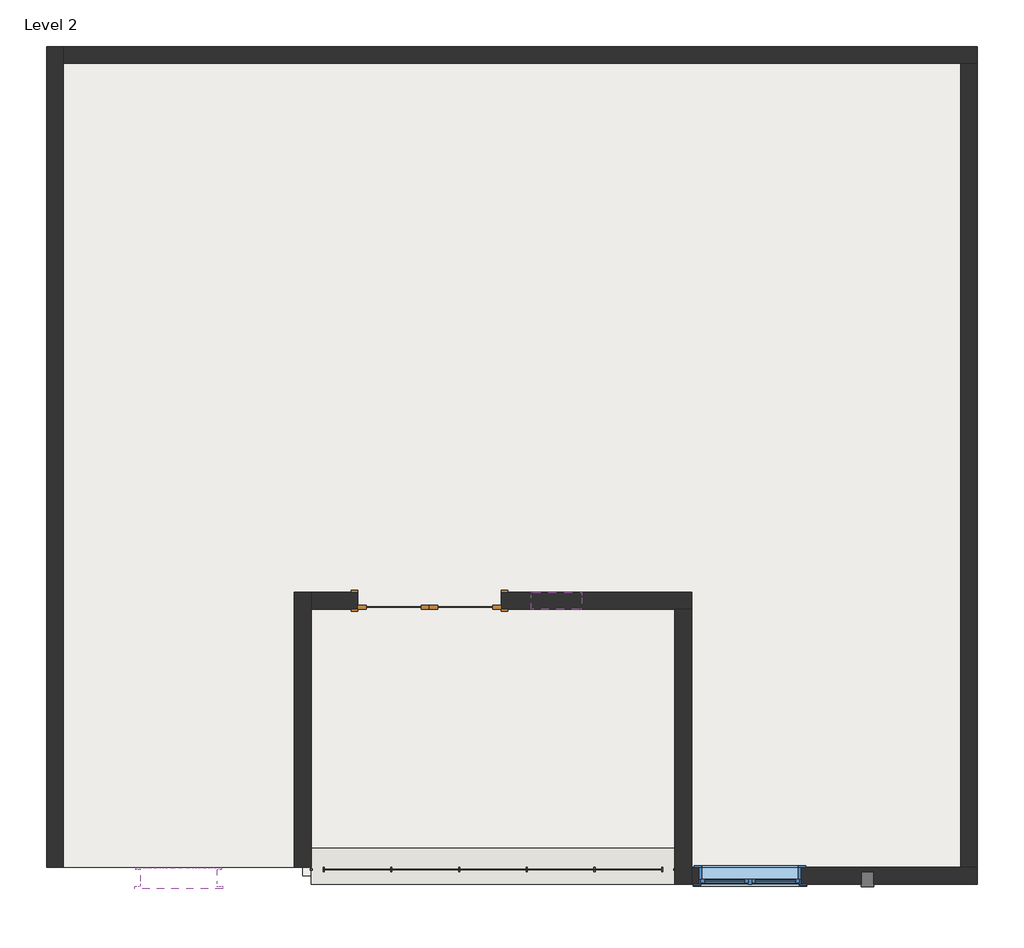
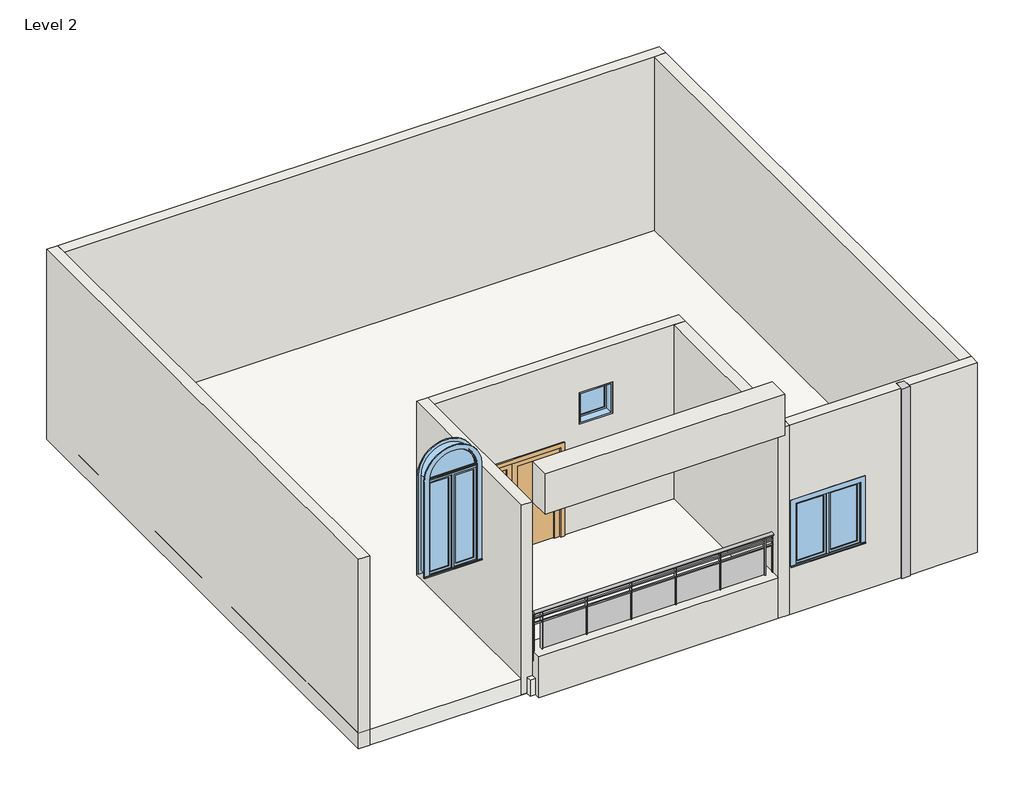
# One storey: 8 walls, 3 windows, 1 door, 1 proxy, 1 railing, 1 roof.
"""IFC4 building model written with IfcOpenShell, lengths in millimetres."""

from ifc_helpers import new_model, si_unit, point, frame, origin, place, context, project, spatial, polyline, ellipse_curve, trimmed, outline, extrude, faceted_brep, transform, mapped, element, save
from ifc_brep_helpers import plane_surface, extruded_surface, advanced_brep
from components import door_10418eaf, walls_4_walls_4_ee6bbb79, window_4e95f2a8, window_0862ab64, window_6846e476

model = new_model("IFC4")

# Units and contexts
model_context = context("Model", 3, world=origin())
ifc_project = project(units=[si_unit("LENGTHUNIT", "METRE", prefix="MILLI")], contexts=[model_context])

# Site, building, storey
site = spatial("IfcSite", under=ifc_project)
building = spatial("IfcBuilding", under=site)
storey = spatial("IfcBuildingStorey", under=building, Name="Level 2", Elevation=3657.6)

# Proxy
placement = place(None, origin())
element("IfcBuildingElementProxy", 1, Name="Reveal", ObjectType="Reveal", at=placement, inside=storey, context=model_context, shape_type="SweptSolid", body=[
    extrude(outline(polyline([(752.5001186, 242.2810824), (752.5001186, 425.1610824), (904.9001186, 425.1610824), (904.9001186, 242.2810824), (752.5001186, 242.2810824)])), frame((0.0, 0.0, 3657.6), z_axis=(0.0, 0.0, 1.0), x_axis=(1.0, 0.0, 0.0)), (0.0, 0.0, 1.0), 3657.6),
])

# Door
door_shape = door_10418eaf(model_context)
element("IfcDoor", 2, ObjectType="Door-Double-Glass : 68\" x 80\"", at=placement, inside=storey, context=model_context, shape_type="MappedRepresentation", body=[
    mapped(door_shape, transform((-4429.0998814, 3678.7423324, 3657.6), x_axis=(-1.0, 0.0, 0.0), y_axis=(0.0, -1.0, 0.0), z_axis=(0.0, 0.0, 1.0))),
])

# Railing
element("IfcRailing", 3, ObjectType="Glass Panel - Bottom Fill", at=placement, inside=storey, context=model_context, shape_type="SolidModel", body=[
    advanced_brep(
    [(-5851.4998814, 488.6610824, 5181.6), (-5851.4998814, 412.4610824, 5181.6), (-1482.6998814, 488.6610824, 5181.6), (-1482.6998814, 412.4610824, 5181.6)],
    [
        (0, 1, ellipse_curve(frame((-5851.4998814, 450.5610824, 5181.6), z_axis=(-1.0, 0.0, 0.0), x_axis=(0.0, -1.0, 0.0)), 38.1, 28.575)),
        (1, 0, ellipse_curve(frame((-5851.4998814, 450.5610824, 5181.6), z_axis=(-1.0, 0.0, 0.0), x_axis=(0.0, -1.0, 0.0)), 38.1, 28.575)),
        (2, 3, ellipse_curve(frame((-1482.6998814, 450.5610824, 5181.6), z_axis=(1.0, 0.0, 0.0), x_axis=(0.0, -1.0, 0.0)), 38.1, 28.575)),
        (3, 2, ellipse_curve(frame((-1482.6998814, 450.5610824, 5181.6), z_axis=(1.0, 0.0, 0.0), x_axis=(0.0, -1.0, 0.0)), 38.1, 28.575)),
        (0, 2),
        (3, 1),
    ],
    [
        plane_surface(frame((-5851.4998814, 450.5610824, 5181.6), z_axis=(-1.0, 0.0, 0.0), x_axis=(0.0, 1.0, 0.0))),
        plane_surface(frame((-1482.6998814, 450.5610824, 5181.6), z_axis=(1.0, 0.0, 0.0), x_axis=(0.0, 1.0, 0.0))),
        extruded_surface(trimmed(ellipse_curve(frame((-1482.6998814, 450.5610824, 5181.6), z_axis=(-1.0, 0.0, 0.0), x_axis=(0.0, -1.0, 0.0)), 38.1, 28.575), [point((-1482.6998814, 488.6610824, 5181.6))], [point((-1482.6998814, 412.4610824, 5181.6))], True, "CARTESIAN"), (-4368.8, 0.0, 0.0), 4368.8),
        extruded_surface(trimmed(ellipse_curve(frame((-1482.6998814, 450.5610824, 5181.6), z_axis=(-1.0, 0.0, 0.0), x_axis=(0.0, -1.0, 0.0)), 38.1, 28.575), [point((-1482.6998814, 412.4610824, 5181.6))], [point((-1482.6998814, 488.6610824, 5181.6))], True, "CARTESIAN"), (-4368.8, 0.0, 0.0), 4368.8),
    ],
    [
        (0, [[1, 2]]),
        (1, [[3, 4]]),
        (2, [[-1, 5, -4, 6]]),
        (3, [[-2, -6, -3, -5]]),
    ],
),
    extrude(outline(polyline([(-5851.4998814, 437.8610824), (-5851.4998814, 463.2610824), (-1482.6998814, 463.2610824), (-1482.6998814, 437.8610824), (-5851.4998814, 437.8610824)])), frame((0.0, 0.0, 5067.3), z_axis=(0.0, 0.0, 1.0), x_axis=(1.0, 0.0, 0.0)), (0.0, 0.0, 1.0), 25.4),
    extrude(outline(polyline([(-5851.4998814, 437.8610824), (-5851.4998814, 463.2610824), (-1482.6998814, 463.2610824), (-1482.6998814, 437.8610824), (-5851.4998814, 437.8610824)])), frame((0.0, 0.0, 4965.7), z_axis=(0.0, 0.0, 1.0), x_axis=(1.0, 0.0, 0.0)), (0.0, 0.0, 1.0), 25.4),
    extrude(outline(polyline([(-1641.4498814, 425.1610824), (-1641.4498814, 475.9610824), (-1628.7498814, 475.9610824), (-1628.7498814, 425.1610824), (-1641.4498814, 425.1610824)])), frame((0.0, 0.0, 4267.2), z_axis=(0.0, 0.0, 1.0), x_axis=(1.0, 0.0, 0.0)), (0.0, 0.0, 1.0), 885.6788223),
    extrude(outline(polyline([(-2447.8998814, 457.0962394), (-1635.0998814, 457.0962394), (-1635.0998814, 450.7462394), (-2447.8998814, 450.7462394), (-2447.8998814, 457.0962394)])), frame((0.0, 0.0, 4368.8), z_axis=(0.0, 0.0, 1.0), x_axis=(1.0, 0.0, 0.0)), (0.0, 0.0, 1.0), 596.9),
    extrude(outline(polyline([(-2454.2498814, 425.1610824), (-2454.2498814, 475.9610824), (-2441.5498814, 475.9610824), (-2441.5498814, 425.1610824), (-2454.2498814, 425.1610824)])), frame((0.0, 0.0, 4267.2), z_axis=(0.0, 0.0, 1.0), x_axis=(1.0, 0.0, 0.0)), (0.0, 0.0, 1.0), 885.6788223),
    extrude(outline(polyline([(-3260.6998814, 457.0962394), (-2447.8998814, 457.0962394), (-2447.8998814, 450.7462394), (-3260.6998814, 450.7462394), (-3260.6998814, 457.0962394)])), frame((0.0, 0.0, 4368.8), z_axis=(0.0, 0.0, 1.0), x_axis=(1.0, 0.0, 0.0)), (0.0, 0.0, 1.0), 596.9),
    extrude(outline(polyline([(-3267.0498814, 425.1610824), (-3267.0498814, 475.9610824), (-3254.3498814, 475.9610824), (-3254.3498814, 425.1610824), (-3267.0498814, 425.1610824)])), frame((0.0, 0.0, 4267.2), z_axis=(0.0, 0.0, 1.0), x_axis=(1.0, 0.0, 0.0)), (0.0, 0.0, 1.0), 885.6788223),
    extrude(outline(polyline([(-4073.4998814, 457.0962394), (-3260.6998814, 457.0962394), (-3260.6998814, 450.7462394), (-4073.4998814, 450.7462394), (-4073.4998814, 457.0962394)])), frame((0.0, 0.0, 4368.8), z_axis=(0.0, 0.0, 1.0), x_axis=(1.0, 0.0, 0.0)), (0.0, 0.0, 1.0), 596.9),
    extrude(outline(polyline([(-4079.8498814, 425.1610824), (-4079.8498814, 475.9610824), (-4067.1498814, 475.9610824), (-4067.1498814, 425.1610824), (-4079.8498814, 425.1610824)])), frame((0.0, 0.0, 4267.2), z_axis=(0.0, 0.0, 1.0), x_axis=(1.0, 0.0, 0.0)), (0.0, 0.0, 1.0), 885.6788223),
    extrude(outline(polyline([(-4886.2998814, 457.0962394), (-4073.4998814, 457.0962394), (-4073.4998814, 450.7462394), (-4886.2998814, 450.7462394), (-4886.2998814, 457.0962394)])), frame((0.0, 0.0, 4368.8), z_axis=(0.0, 0.0, 1.0), x_axis=(1.0, 0.0, 0.0)), (0.0, 0.0, 1.0), 596.9),
    extrude(outline(polyline([(-4892.6498814, 425.1610824), (-4892.6498814, 475.9610824), (-4879.9498814, 475.9610824), (-4879.9498814, 425.1610824), (-4892.6498814, 425.1610824)])), frame((0.0, 0.0, 4267.2), z_axis=(0.0, 0.0, 1.0), x_axis=(1.0, 0.0, 0.0)), (0.0, 0.0, 1.0), 885.6788223),
    extrude(outline(polyline([(-5699.0998814, 457.0962394), (-4886.2998814, 457.0962394), (-4886.2998814, 450.7462394), (-5699.0998814, 450.7462394), (-5699.0998814, 457.0962394)])), frame((0.0, 0.0, 4368.8), z_axis=(0.0, 0.0, 1.0), x_axis=(1.0, 0.0, 0.0)), (0.0, 0.0, 1.0), 596.9),
    extrude(outline(polyline([(-5705.4498814, 425.1610824), (-5705.4498814, 475.9610824), (-5692.7498814, 475.9610824), (-5692.7498814, 425.1610824), (-5705.4498814, 425.1610824)])), frame((0.0, 0.0, 4267.2), z_axis=(0.0, 0.0, 1.0), x_axis=(1.0, 0.0, 0.0)), (0.0, 0.0, 1.0), 885.6788223),
    extrude(outline(polyline([(-1495.3998814, 441.0360824), (-1495.3998814, 460.0860824), (-1476.3498814, 460.0860824), (-1476.3498814, 441.0360824), (-1495.3998814, 441.0360824)])), frame((0.0, 0.0, 4267.2), z_axis=(0.0, 0.0, 1.0), x_axis=(1.0, 0.0, 0.0)), (0.0, 0.0, 1.0), 885.6788223),
    extrude(outline(polyline([(-5857.8498814, 441.0360824), (-5857.8498814, 460.0860824), (-5838.7998814, 460.0860824), (-5838.7998814, 441.0360824), (-5857.8498814, 441.0360824)])), frame((0.0, 0.0, 4267.2), z_axis=(0.0, 0.0, 1.0), x_axis=(1.0, 0.0, 0.0)), (0.0, 0.0, 1.0), 885.6788223),
])

# Roof
element("IfcRoof", 4, ObjectType="Generic - 12\"", at=placement, inside=storey, context=model_context, shape_type="SweptSolid", body=[
    extrude(outline(polyline([(-9026.4998814, 10331.1610824), (2149.5001186, 10331.1610824), (2149.5001186, 374.3610824), (-5953.0998814, 374.3610824), (-5953.0998814, 475.9610824), (-9026.4998814, 475.9610824), (-9026.4998814, 10331.1610824)])), frame((0.0, 0.0, 3657.6), z_axis=(0.0, 0.0, 1.0), x_axis=(1.0, 0.0, 0.0)), (0.0, 0.0, 1.0), 304.8),
])

# Walls
element("IfcWall", 5, ObjectType="Generic - 8\"", at=placement, inside=storey, context=model_context, shape_type="Brep", body=[
    faceted_brep([(-5851.4998814, 475.9610824, 3657.6), (-5851.4998814, 3574.7610824, 3657.6), (-5851.4998814, 3777.9610824, 3657.6), (-5851.4998814, 3777.9610824, 7315.2), (-5851.4998814, 3574.7610824, 7315.2), (-5851.4998814, 475.9610824, 7315.2), (-6054.6998814, 475.9610824, 3657.6), (-6054.6998814, 475.9610824, 7315.2), (-6054.6998814, 3777.9610824, 7315.2), (-6054.6998814, 3777.9610824, 3657.6)], [[[0, 1, 2, 3, 4, 5]], [[6, 7, 8, 9]], [[2, 1, 0, 6, 9]], [[5, 4, 3, 8, 7]], [[0, 5, 7, 6]], [[3, 2, 9, 8]]]),
])
element("IfcWall", 6, ObjectType="Generic - 8\"", at=placement, inside=storey, context=model_context, shape_type="Brep", body=[
    faceted_brep([(-5851.4998814, 3574.7610824, 3657.6), (-5292.6998814, 3574.7610824, 3657.6), (-5292.6998814, 3574.7610824, 5689.6), (-3565.4998814, 3574.7610824, 5689.6), (-3565.4998814, 3574.7610824, 3657.6), (-1482.6998814, 3574.7610824, 3657.6), (-1279.4998814, 3574.7610824, 3657.6), (-1279.4998814, 3574.7610824, 7315.2), (-1482.6998814, 3574.7610824, 7315.2), (-5851.4998814, 3574.7610824, 7315.2), (-2600.2998814, 3574.7610824, 6609.4918678), (-2600.2998814, 3574.7610824, 5999.8918678), (-3209.8998814, 3574.7610824, 5999.8918678), (-3209.8998814, 3574.7610824, 6609.4918678), (-5292.6998814, 3777.9610824, 5689.6), (-5292.6998814, 3777.9610824, 3657.6), (-5851.4998814, 3777.9610824, 3657.6), (-5851.4998814, 3777.9610824, 7315.2), (-1279.4998814, 3777.9610824, 7315.2), (-1279.4998814, 3777.9610824, 3657.6), (-3565.4998814, 3777.9610824, 3657.6), (-3565.4998814, 3777.9610824, 5689.6), (-2600.2998814, 3777.9610824, 6609.4918678), (-3209.8998814, 3777.9610824, 6609.4918678), (-3209.8998814, 3777.9610824, 5999.8918678), (-2600.2998814, 3777.9610824, 5999.8918678)], [[[0, 1, 2, 3, 4, 5, 6, 7, 8, 9], [10, 11, 12, 13]], [[14, 15, 16, 17, 18, 19, 20, 21], [22, 23, 24, 25]], [[20, 19, 6, 5, 4]], [[16, 15, 1, 0]], [[9, 8, 7, 18, 17]], [[0, 9, 17, 16]], [[7, 6, 19, 18]], [[11, 10, 22, 25]], [[12, 11, 25, 24]], [[13, 12, 24, 23]], [[10, 13, 23, 22]], [[2, 1, 15, 14]], [[3, 2, 14, 21]], [[4, 3, 21, 20]]]),
])
element("IfcWall", 7, ObjectType="Generic - 8\"", at=placement, inside=storey, context=model_context, shape_type="Brep", body=[
    faceted_brep([(-1482.6998814, 3574.7610824, 3657.6), (-1482.6998814, 272.7610824, 3657.6), (-1482.6998814, 272.7610824, 7315.2), (-1482.6998814, 3574.7610824, 7315.2), (-1279.4998814, 3574.7610824, 3657.6), (-1279.4998814, 3574.7610824, 7315.2), (-1279.4998814, 475.9610824, 7315.2), (-1279.4998814, 272.7610824, 7315.2), (-1279.4998814, 272.7610824, 3657.6), (-1279.4998814, 475.9610824, 3657.6)], [[[0, 1, 2, 3]], [[4, 5, 6, 7, 8, 9]], [[1, 0, 4, 9, 8]], [[3, 2, 7, 6, 5]], [[0, 3, 5, 4]], [[2, 1, 8, 7]]]),
])
element("IfcWall", 8, ObjectType="Generic - 8\"", at=placement, inside=storey, context=model_context, shape_type="Brep", body=[
    faceted_brep([(-1279.4998814, 272.7610824, 7315.2), (-1279.4998814, 272.7610824, 3657.6), (752.5001186, 272.7610824, 3657.6), (752.5001186, 272.7610824, 7315.2), (-1190.5998814, 272.7610824, 4572.0), (-1190.5998814, 272.7610824, 5791.2), (28.6001186, 272.7610824, 5791.2), (28.6001186, 272.7610824, 4572.0), (2149.5001186, 272.7610824, 3657.6), (2149.5001186, 272.7610824, 7315.2), (904.9001186, 272.7610824, 7315.2), (904.9001186, 272.7610824, 3657.6), (1539.9001186, 272.7610824, 3657.6), (2149.5001186, 475.9610824, 3657.6), (1946.3001186, 475.9610824, 3657.6), (-1279.4998814, 475.9610824, 3657.6), (-1279.4998814, 475.9610824, 7315.2), (1946.3001186, 475.9610824, 7315.2), (2149.5001186, 475.9610824, 7315.2), (-1190.5998814, 475.9610824, 5791.2), (-1190.5998814, 475.9610824, 4572.0), (28.6001186, 475.9610824, 4572.0), (28.6001186, 475.9610824, 5791.2), (904.9001186, 425.1610824, 3657.6), (752.5001186, 425.1610824, 3657.6), (752.5001186, 425.1610824, 7315.2), (904.9001186, 425.1610824, 7315.2)], [[[0, 1, 2, 3], [4, 5, 6, 7]], [[8, 9, 10, 11, 12]], [[13, 14, 15, 16, 17, 18], [19, 20, 21, 22]], [[15, 14, 13, 8, 12, 11, 23, 24, 2, 1]], [[18, 17, 16, 0, 3, 25, 26, 10, 9]], [[1, 0, 16, 15]], [[9, 8, 13, 18]], [[20, 19, 5, 4]], [[21, 20, 4, 7]], [[22, 21, 7, 6]], [[19, 22, 6, 5]], [[26, 23, 11, 10]], [[23, 26, 25, 24]], [[24, 25, 3, 2]]]),
])
element("IfcWall", 9, ObjectType="Generic - 8\"", at=placement, inside=storey, context=model_context, shape_type="Brep", body=[
    faceted_brep([(-8823.2998814, 475.9610824, 3657.6), (-8823.2998814, 10127.9610824, 3657.6), (-8823.2998814, 10331.1610824, 3657.6), (-8823.2998814, 10331.1610824, 7315.2), (-8823.2998814, 10127.9610824, 7315.2), (-8823.2998814, 475.9610824, 7315.2), (-9026.4998814, 475.9610824, 3657.6), (-9026.4998814, 475.9610824, 7315.2), (-9026.4998814, 10331.1610824, 7315.2), (-9026.4998814, 10331.1610824, 3657.6)], [[[0, 1, 2, 3, 4, 5]], [[6, 7, 8, 9]], [[2, 1, 0, 6, 9]], [[5, 4, 3, 8, 7]], [[0, 5, 7, 6]], [[3, 2, 9, 8]]]),
])
element("IfcWall", 10, ObjectType="Generic - 8\"", at=placement, inside=storey, context=model_context, shape_type="Brep", body=[
    faceted_brep([(-8823.2998814, 10127.9610824, 3657.6), (1946.3001186, 10127.9610824, 3657.6), (2149.5001186, 10127.9610824, 3657.6), (2149.5001186, 10127.9610824, 7315.2), (1946.3001186, 10127.9610824, 7315.2), (-8823.2998814, 10127.9610824, 7315.2), (-8823.2998814, 10331.1610824, 3657.6), (-8823.2998814, 10331.1610824, 7315.2), (2149.5001186, 10331.1610824, 7315.2), (2149.5001186, 10331.1610824, 3657.6), (1539.9001186, 10331.1610824, 3657.6)], [[[0, 1, 2, 3, 4, 5]], [[6, 7, 8, 9, 10]], [[2, 1, 0, 6, 10, 9]], [[5, 4, 3, 8, 7]], [[0, 5, 7, 6]], [[3, 2, 9, 8]]]),
])
element("IfcWall", 11, ObjectType="Generic - 8\"", at=placement, inside=storey, context=model_context, shape_type="Brep", body=[
    faceted_brep([(1946.3001186, 10127.9610824, 3657.6), (1946.3001186, 475.9610824, 3657.6), (1946.3001186, 475.9610824, 7315.2), (1946.3001186, 10127.9610824, 7315.2), (2149.5001186, 10127.9610824, 3657.6), (2149.5001186, 10127.9610824, 7315.2), (2149.5001186, 475.9610824, 7315.2), (2149.5001186, 475.9610824, 3657.6), (2149.5001186, 882.3610824, 3657.6), (2149.5001186, 4590.7610824, 3657.6), (2149.5001186, 5200.3610824, 3657.6), (2149.5001186, 9721.5610824, 3657.6)], [[[0, 1, 2, 3]], [[4, 5, 6, 7, 8, 9, 10, 11]], [[1, 0, 4, 11, 10, 9, 8, 7]], [[3, 2, 6, 5]], [[2, 1, 7, 6]], [[0, 3, 5, 4]]]),
])
walls_4_walls_4_shape = walls_4_walls_4_ee6bbb79(model_context)
element("IfcWall", 12, ObjectType="Walls 4 : Walls 4", at=placement, inside=storey, context=model_context, shape_type="MappedRepresentation", body=[
    mapped(walls_4_walls_4_shape, transform((0.0, 0.0, 0.0), x_axis=(1.0, 0.0, 0.0), y_axis=(0.0, 1.0, 0.0), z_axis=(0.0, 0.0, 1.0))),
])

# Windows
window_shape = window_4e95f2a8(model_context)
element("IfcWindow", 13, ObjectType="36\" x 72\"", at=placement, inside=storey, context=model_context, shape_type="MappedRepresentation", body=[
    mapped(window_shape, transform((-7430.9977233, 348.9610824, 6415.9920702), x_axis=(-1.0, 0.0, 0.0), y_axis=(0.0, -1.0, 0.0), z_axis=(0.0, 0.0, 1.0))),
])
window_2_shape = window_0862ab64(model_context)
element("IfcWindow", 14, ObjectType="Casement Dbl with Trim.0001 : 48\" x 48\"", at=placement, inside=storey, context=model_context, shape_type="MappedRepresentation", body=[
    mapped(window_2_shape, transform((-580.9998814, 393.4110824, 3657.6), x_axis=(-1.0, 0.0, 0.0), y_axis=(0.0, -1.0, 0.0), z_axis=(0.0, 0.0, 1.0))),
])
window_3_shape = window_6846e476(model_context)
element("IfcWindow", 15, ObjectType="Fixed : 24\" x 24\"", at=placement, inside=storey, context=model_context, shape_type="MappedRepresentation", body=[
    mapped(window_3_shape, transform((-2866.9998814, 3676.3610824, 5085.4918678), x_axis=(1.0, 0.0, 0.0), y_axis=(0.0, 1.0, 0.0), z_axis=(0.0, 0.0, 1.0))),
])

save(model, "model.ifc")

# Revit data of these elements
# Type "Door-Double-Glass : 68\" x 80\""
#   Type Mark = "8"
#   Construction Type Id = "opn-d45"
#   Assembly Code = "C1020"
#   Analytic Construction = "Wood frame, double glass door "
#   W = 2' - 10"
#   Thickness = 0' - 2"
#   Thermal Resistance (R) = 1.8150 (h·ft²·°F)/BTU
#   Swing Angle [instance default] = 90.00°
#   Heat Transfer Coefficient (U) = 0.5510 BTU/(h·ft²·°F)
#   Height = 6' - 8"
#   Bottom Rail = 0' - 4"
#   Top Rail = 0' - 4"
#   Stiles = 0' - 4"
#   Trim Projection = 0' - 1"
#   Trim Width = 0' - 3"
#   Width = 5' - 8"
#   Define Thermal Properties by = 1
#   Glazing = Glass
#   Panel Material = Wood - Birch - Solid Stained Light Low Gloss
#   Trim Material = Paint - Sienna
#   Visual Light Transmittance = 0
#   Solar Heat Gain Coefficient = 0
#   Function = (empty or 0)
#   Wall Closure = (empty or 0)
# Type "Glass Panel - Bottom Fill"
#   Assembly Code = "C2010400"
#   built-in parameter 1008612 = 0.0416667 (stored number, unit not read)
#   built-in parameter 1008611 = 0.0416667 (stored number, unit not read)
#   built-in parameter 1008609 = 0.333333 (stored number, unit not read)
#   built-in parameter 1008604 = 0.166667 (stored number, unit not read)
#   built-in parameter 1008603 = 0.166667 (stored number, unit not read)
#   Railing Height = 3' - 0"
#   built-in parameter 1008630 = 2
#   built-in parameter 1008610 = 2
#   built-in parameter 1008618 = Baluster - Square : 3/4"
# Type "Generic - 12\""
#   Assembly Code = "B1020"
#   Layers, outside or top first: 1' - 0" no material (function 1)
# Type "Generic - 8\""
#   Assembly Code = "B2010"
#   Layers, outside or top first: 0' - 8" no material (function 1)
# Type "36\" x 72\""
#   Type Mark = "10"
#   Construction Type Id = "SGL"
#   Assembly Code = "B2020100"
#   Analytic Construction = "Large single-glazed windows"
#   Visual Light Transmittance = 0.9
#   Solar Heat Gain Coefficient = 0.86
#   Heat Transfer Coefficient (U) = 0.979472 BTU/(h·ft²·°F)
#   Height = 6' - 0"
#   Default Sill Height = 1' - 0"
#   Trim Projection - Ext. = 0' - 0 1/2"
#   Trim Projection - Int. = 0' - 0 3/4"
#   Trim Width - Exterior = 0' - 3 1/2"
#   Trim Width - Interior = 0' - 3 1/2"
#   Width = 3' - 0"
#   Window Inset = 0' - 0 3/4"
#   Define Thermal Properties by = 1
#   Glass Pane Material = Glass
#   Sash Material = Sash
#   Trim Exterior Material = Trim
#   Trim Interior Material = Trim
#   Wall Closure = (empty or 0)
# Type "Casement Dbl with Trim.0001 : 48\" x 48\""
#   Type Mark = "14"
#   Construction Type Id = "GSP4R"
#   Assembly Code = "B2020100"
#   Analytic Construction = "1/8 in Pilkington single glazing"
#   Visual Light Transmittance = 0.9
#   Solar Heat Gain Coefficient = 0.78
#   Heat Transfer Coefficient (U) = 0.6496 BTU/(h·ft²·°F)
#   Height = 4' - 0"
#   Default Sill Height = 3' - 0"
#   Trim Projection - Ext. = 0' - 0 1/2"
#   Trim Projection - Int. = 0' - 0 3/4"
#   Trim Width - Exterior = 0' - 3 1/2"
#   Trim Width - Interior = 0' - 3 1/2"
#   Width = 4' - 0"
#   Window Inset = 0' - 0 3/4"
#   Define Thermal Properties by = 1
#   Glass Pane Material = Glass
#   Sash Material = Sash
#   Trim Exterior Material = Trim
#   Trim Interior Material = Trim
#   Wall Closure = (empty or 0)
# Type "Fixed : 24\" x 24\""
#   Type Mark = "3"
#   Construction Type Id = "GSP4R"
#   Assembly Code = "B2020100"
#   Analytic Construction = "1/8 in Pilkington single glazing"
#   Visual Light Transmittance = 0.9
#   Solar Heat Gain Coefficient = 0.78
#   Heat Transfer Coefficient (U) = 0.6496 BTU/(h·ft²·°F)
#   Height = 2' - 0"
#   Default Sill Height = 3' - 0"
#   Width = 2' - 0"
#   Window Inset = 0' - 0 3/4"
#   Define Thermal Properties by = 1
#   Glass Pane Material = Glass
#   Sash Material = Sash
#   Wall Closure = (empty or 0)
# Element 2 (IfcDoor, "Door-Double-Glass : 68\" x 80\"")
#   Swing Angle = 90.00°
#   Phase Created = New Construction
#   Materials on its faces: "Wood - Birch - Solid Stained Light Low Gloss", "Paint - Sienna", "Glass"
# Element 3 (IfcRailing, "Glass Panel - Bottom Fill")
#   built-in parameter 1008621 = 2 (stored number, unit not read)
#   Phase Created = New Construction
#   Materials on its faces: "Glass"
# Element 4 (IfcRoof, "Generic - 12\"")
#   built-in parameter 1001705 = 13 (stored number, unit not read)
#   built-in parameter 1001710 = 33615
#   Phase Created = New Construction
#   Materials on its faces: "Default Roof"
# Elements 5, 6, 7, 8, 9, 10, 11 (IfcWall, "Generic - 8\"")
#   Top Offset = 0' - 0"
#   Base Offset = 0' - 0"
#   Unconnected Height = 12' - 0"
#   wall height = 12' - 0"
#   Phase Created = New Construction
#   Base Constraint = Level 2
#   Materials on its faces: "Default Wall"
# Element 12 (IfcWall, "Walls 4 : Walls 4")
#   Phase Created = New Construction
#   Materials on its faces: "Default Wall"
# Element 13 (IfcWindow, "36\" x 72\"")
#   Mark = "1"
#   Phase Created = New Construction
#   Materials on its faces: "Sash", "Trim", "Glass"
# Element 14 (IfcWindow, "Casement Dbl with Trim.0001 : 48\" x 48\"")
#   Mark = "5"
#   Phase Created = New Construction
#   Materials on its faces: "Sash", "Trim", "Glass"
# Element 15 (IfcWindow, "Fixed : 24\" x 24\"")
#   Mark = "8"
#   Phase Created = New Construction
#   Materials on its faces: "Sash", "Glass"
# Materials
#   "Glass": class "Glass", colour RGB 0 128 192, transparency 0.75, Description = "Soda Lime Glass", Cost = 0
#   "Wood - Birch - Solid Stained Light Low Gloss": class "Wood", colour RGB 210 159 95, transparency 0, Cost = 0
#   "Paint - Sienna": colour RGB 118 70 51, transparency 0, Cost = 0
#   "Sash": class "Wood", colour RGB 224 178 126, transparency 0
#   "Trim": class "Wood", colour RGB 224 178 126, transparency 0
#   "Default Roof": colour RGB 88 101 114, transparency 0
#   "Default Wall": colour RGB 128 128 128, transparency 0
